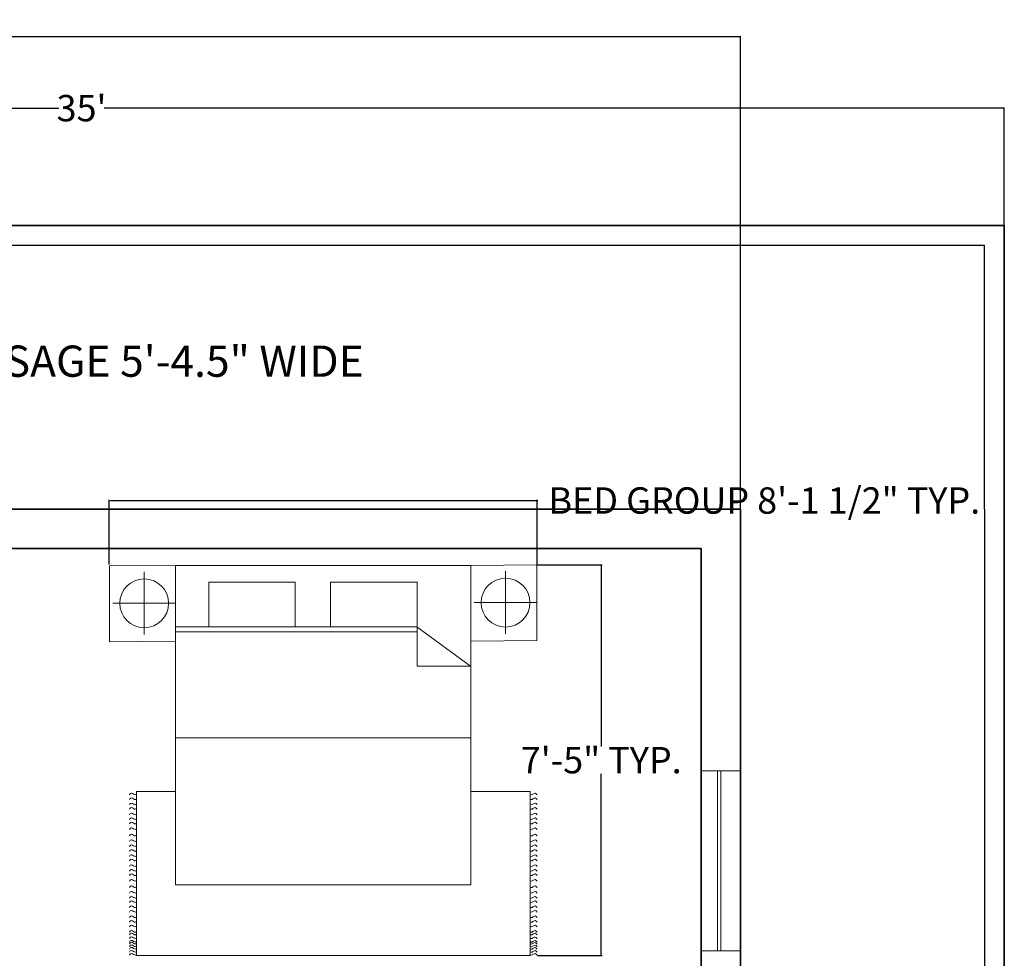
# Model space of a CAD drawing. Units: inches. Extents: x 79 to 8696167, y -3690578 to 147.
# Tile 7 of 10: x 329 to 553, y -67 to 147. Entities that reach past the tile are written whole.
import ezdxf

# ---------------------------------------------------------------- set-up
doc = ezdxf.new("R2010")
doc.units = ezdxf.units.IN
doc.header["$MEASUREMENT"] = 0
doc.layers.get('0').update_dxf_attribs({"color": 253})
for name, color, linetype, lineweight in [('A-ANNO-DIMS', 2, 'Continuous', 18), ('A-AREA-IDEN', 7, 'Continuous', 18), ('C-PROP', 7, 'Continuous', 35), ('C-SITE-WALL', 8, 'Continuous', 25), ('furniture', 30, 'Continuous', 18), ('walls', 8, 'Continuous', 35), ('windows', 171, 'Continuous', 18)]:
    doc.layers.add(name, color=color, linetype=linetype, lineweight=lineweight)
doc.styles.get("Standard").update_dxf_attribs({"font": 'arial.ttf'})
doc.dimstyles.get("Standard").update_dxf_attribs({"dimtxt": 6, "dimasz": 0.18, "dimexe": 0.18, "dimexo": 0.0625, "dimgap": 0.09, "dimtad": 0, "dimtih": 1, "dimtoh": 1, "dimzin": 0, "dimdsep": 46, "dimlunit": 3, "dimtxsty": 'Standard', "dimcen": 0.09, "dimadec": 0, "dimazin": 0, "dimtfac": 1, "dimtofl": 0, "dimtmove": 0, "dimatfit": 3, "dimfxl": 1, "dimtolj": 1, "dimtzin": 0, "dimarcsym": 0})

# ---------------------------------------------------------------- blocks, each defined once
blk = doc.blocks.new('CARPET')
at = {"layer": 'furniture'}
for p, q in [((-51.53, -98.11), (-51.53, -55.12)), ((-51.53, -55.12), (-41.27, -55.12)), ((36, -55.12), (51.55, -55.12)), ((51.55, -55.12), (51.55, -98.11)), ((51.55, -98.11), (-51.53, -98.11))]:
    blk.add_line(p, q, dxfattribs=at)
for points, knots in [([(-53.37, -55.99), (-53.22, -55.8), (-52.9, -55.41), (-52.34, -55.8), (-51.89, -56.08), (-51.65, -55.91), (-51.53, -55.83)], [0, 0, 0, 0, 0.653278, 1.290138, 1.740457, 2.114451, 2.114451, 2.114451, 2.114451]), ([(53.37, -55.99), (53.22, -55.8), (52.9, -55.41), (52.34, -55.8), (51.89, -56.08), (51.65, -55.91), (51.53, -55.83)], [0, 0, 0, 0, 0.653278, 1.290138, 1.740457, 2.114451, 2.114451, 2.114451, 2.114451]), ([(-53.37, -57.26), (-53.22, -57.07), (-52.9, -56.67), (-52.34, -57.07), (-51.89, -57.35), (-51.65, -57.17), (-51.53, -57.1)], [0, 0, 0, 0, 0.653278, 1.290138, 1.740457, 2.114451, 2.114451, 2.114451, 2.114451]), ([(-53.37, -58.59), (-53.22, -58.4), (-52.9, -58.01), (-52.34, -58.4), (-51.89, -58.68), (-51.65, -58.5), (-51.53, -58.43)], [0, 0, 0, 0, 0.653278, 1.290138, 1.740457, 2.114451, 2.114451, 2.114451, 2.114451]), ([(53.37, -57.26), (53.22, -57.07), (52.9, -56.67), (52.34, -57.07), (51.89, -57.35), (51.65, -57.17), (51.53, -57.1)], [0, 0, 0, 0, 0.653278, 1.290138, 1.740457, 2.114451, 2.114451, 2.114451, 2.114451]), ([(53.37, -58.59), (53.22, -58.4), (52.9, -58.01), (52.34, -58.4), (51.89, -58.68), (51.65, -58.5), (51.53, -58.43)], [0, 0, 0, 0, 0.653278, 1.290138, 1.740457, 2.114451, 2.114451, 2.114451, 2.114451]), ([(-53.37, -59.78), (-53.22, -59.58), (-52.9, -59.19), (-52.34, -59.58), (-51.89, -59.86), (-51.65, -59.69), (-51.53, -59.61)], [0, 0, 0, 0, 0.653278, 1.290138, 1.740457, 2.114451, 2.114451, 2.114451, 2.114451]), ([(-53.37, -61.22), (-53.22, -61.02), (-52.9, -60.63), (-52.34, -61.02), (-51.89, -61.3), (-51.65, -61.13), (-51.53, -61.05)], [0, 0, 0, 0, 0.653278, 1.290138, 1.740457, 2.114451, 2.114451, 2.114451, 2.114451]), ([(53.37, -59.78), (53.22, -59.58), (52.9, -59.19), (52.34, -59.58), (51.89, -59.86), (51.65, -59.69), (51.53, -59.61)], [0, 0, 0, 0, 0.653278, 1.290138, 1.740457, 2.114451, 2.114451, 2.114451, 2.114451]), ([(53.37, -61.22), (53.22, -61.02), (52.9, -60.63), (52.34, -61.02), (51.89, -61.3), (51.65, -61.13), (51.53, -61.05)], [0, 0, 0, 0, 0.653278, 1.290138, 1.740457, 2.114451, 2.114451, 2.114451, 2.114451]), ([(-53.37, -62.44), (-53.22, -62.25), (-52.9, -61.86), (-52.34, -62.25), (-51.89, -62.53), (-51.65, -62.36), (-51.53, -62.28)], [0, 0, 0, 0, 0.653278, 1.290138, 1.740457, 2.114451, 2.114451, 2.114451, 2.114451]), ([(-53.37, -63.63), (-53.22, -63.43), (-52.9, -63.04), (-52.34, -63.43), (-51.89, -63.72), (-51.65, -63.54), (-51.53, -63.46)], [0, 0, 0, 0, 0.653278, 1.290138, 1.740457, 2.114451, 2.114451, 2.114451, 2.114451]), ([(53.37, -62.44), (53.22, -62.25), (52.9, -61.86), (52.34, -62.25), (51.89, -62.53), (51.65, -62.36), (51.53, -62.28)], [0, 0, 0, 0, 0.653278, 1.290138, 1.740457, 2.114451, 2.114451, 2.114451, 2.114451]), ([(53.37, -63.63), (53.22, -63.43), (52.9, -63.04), (52.34, -63.43), (51.89, -63.72), (51.65, -63.54), (51.53, -63.46)], [0, 0, 0, 0, 0.653278, 1.290138, 1.740457, 2.114451, 2.114451, 2.114451, 2.114451]), ([(-53.37, -65.07), (-53.22, -64.87), (-52.9, -64.48), (-52.34, -64.87), (-51.89, -65.15), (-51.65, -64.98), (-51.53, -64.9)], [0, 0, 0, 0, 0.653278, 1.290138, 1.740457, 2.114451, 2.114451, 2.114451, 2.114451]), ([(-53.37, -66.76), (-53.22, -66.56), (-52.9, -66.17), (-52.34, -66.56), (-51.89, -66.84), (-51.65, -66.67), (-51.53, -66.59)], [0, 0, 0, 0, 0.653278, 1.290138, 1.740457, 2.114451, 2.114451, 2.114451, 2.114451]), ([(53.37, -65.07), (53.22, -64.87), (52.9, -64.48), (52.34, -64.87), (51.89, -65.15), (51.65, -64.98), (51.53, -64.9)], [0, 0, 0, 0, 0.653278, 1.290138, 1.740457, 2.114451, 2.114451, 2.114451, 2.114451]), ([(53.37, -66.76), (53.22, -66.56), (52.9, -66.17), (52.34, -66.56), (51.89, -66.84), (51.65, -66.67), (51.53, -66.59)], [0, 0, 0, 0, 0.653278, 1.290138, 1.740457, 2.114451, 2.114451, 2.114451, 2.114451]), ([(-53.37, -68.2), (-53.22, -68), (-52.9, -67.61), (-52.34, -68), (-51.89, -68.28), (-51.65, -68.11), (-51.53, -68.03)], [0, 0, 0, 0, 0.653278, 1.290138, 1.740457, 2.114451, 2.114451, 2.114451, 2.114451]), ([(-53.37, -69.53), (-53.22, -69.33), (-52.9, -68.94), (-52.34, -69.33), (-51.89, -69.61), (-51.65, -69.44), (-51.53, -69.36)], [0, 0, 0, 0, 0.653278, 1.290138, 1.740457, 2.114451, 2.114451, 2.114451, 2.114451]), ([(53.37, -68.2), (53.22, -68), (52.9, -67.61), (52.34, -68), (51.89, -68.28), (51.65, -68.11), (51.53, -68.03)], [0, 0, 0, 0, 0.653278, 1.290138, 1.740457, 2.114451, 2.114451, 2.114451, 2.114451]), ([(53.37, -69.53), (53.22, -69.33), (52.9, -68.94), (52.34, -69.33), (51.89, -69.61), (51.65, -69.44), (51.53, -69.36)], [0, 0, 0, 0, 0.653278, 1.290138, 1.740457, 2.114451, 2.114451, 2.114451, 2.114451]), ([(-53.37, -70.79), (-53.22, -70.6), (-52.9, -70.21), (-52.34, -70.6), (-51.89, -70.88), (-51.65, -70.7), (-51.53, -70.63)], [0, 0, 0, 0, 0.653278, 1.290138, 1.740457, 2.114451, 2.114451, 2.114451, 2.114451]), ([(-53.37, -72.12), (-53.22, -71.93), (-52.9, -71.54), (-52.34, -71.93), (-51.89, -72.21), (-51.65, -72.04), (-51.53, -71.96)], [0, 0, 0, 0, 0.653278, 1.290138, 1.740457, 2.114451, 2.114451, 2.114451, 2.114451]), ([(53.37, -70.79), (53.22, -70.6), (52.9, -70.21), (52.34, -70.6), (51.89, -70.88), (51.65, -70.7), (51.53, -70.63)], [0, 0, 0, 0, 0.653278, 1.290138, 1.740457, 2.114451, 2.114451, 2.114451, 2.114451]), ([(53.37, -72.12), (53.22, -71.93), (52.9, -71.54), (52.34, -71.93), (51.89, -72.21), (51.65, -72.04), (51.53, -71.96)], [0, 0, 0, 0, 0.653278, 1.290138, 1.740457, 2.114451, 2.114451, 2.114451, 2.114451]), ([(-53.37, -73.31), (-53.22, -73.11), (-52.9, -72.72), (-52.34, -73.11), (-51.89, -73.4), (-51.65, -73.22), (-51.53, -73.14)], [0, 0, 0, 0, 0.653278, 1.290138, 1.740457, 2.114451, 2.114451, 2.114451, 2.114451]), ([(-53.37, -74.75), (-53.22, -74.55), (-52.9, -74.16), (-52.34, -74.55), (-51.89, -74.83), (-51.65, -74.66), (-51.53, -74.58)], [0, 0, 0, 0, 0.653278, 1.290138, 1.740457, 2.114451, 2.114451, 2.114451, 2.114451]), ([(53.37, -73.31), (53.22, -73.11), (52.9, -72.72), (52.34, -73.11), (51.89, -73.4), (51.65, -73.22), (51.53, -73.14)], [0, 0, 0, 0, 0.653278, 1.290138, 1.740457, 2.114451, 2.114451, 2.114451, 2.114451]), ([(53.37, -74.75), (53.22, -74.55), (52.9, -74.16), (52.34, -74.55), (51.89, -74.83), (51.65, -74.66), (51.53, -74.58)], [0, 0, 0, 0, 0.653278, 1.290138, 1.740457, 2.114451, 2.114451, 2.114451, 2.114451]), ([(-53.37, -75.98), (-53.22, -75.78), (-52.9, -75.39), (-52.34, -75.78), (-51.89, -76.06), (-51.65, -75.89), (-51.53, -75.81)], [0, 0, 0, 0, 0.653278, 1.290138, 1.740457, 2.114451, 2.114451, 2.114451, 2.114451]), ([(-53.37, -77.16), (-53.22, -76.96), (-52.9, -76.57), (-52.34, -76.96), (-51.89, -77.25), (-51.65, -77.07), (-51.53, -76.99)], [0, 0, 0, 0, 0.653278, 1.290138, 1.740457, 2.114451, 2.114451, 2.114451, 2.114451]), ([(53.37, -75.98), (53.22, -75.78), (52.9, -75.39), (52.34, -75.78), (51.89, -76.06), (51.65, -75.89), (51.53, -75.81)], [0, 0, 0, 0, 0.653278, 1.290138, 1.740457, 2.114451, 2.114451, 2.114451, 2.114451]), ([(53.37, -77.16), (53.22, -76.96), (52.9, -76.57), (52.34, -76.96), (51.89, -77.25), (51.65, -77.07), (51.53, -76.99)], [0, 0, 0, 0, 0.653278, 1.290138, 1.740457, 2.114451, 2.114451, 2.114451, 2.114451]), ([(-53.37, -78.6), (-53.22, -78.4), (-52.9, -78.01), (-52.34, -78.4), (-51.89, -78.68), (-51.65, -78.51), (-51.53, -78.43)], [0, 0, 0, 0, 0.653278, 1.290138, 1.740457, 2.114451, 2.114451, 2.114451, 2.114451]), ([(-53.37, -80.29), (-53.22, -80.09), (-52.9, -79.7), (-52.34, -80.09), (-51.89, -80.37), (-51.65, -80.2), (-51.53, -80.12)], [0, 0, 0, 0, 0.653278, 1.290138, 1.740457, 2.114451, 2.114451, 2.114451, 2.114451]), ([(53.37, -78.6), (53.22, -78.4), (52.9, -78.01), (52.34, -78.4), (51.89, -78.68), (51.65, -78.51), (51.53, -78.43)], [0, 0, 0, 0, 0.653278, 1.290138, 1.740457, 2.114451, 2.114451, 2.114451, 2.114451]), ([(53.37, -80.29), (53.22, -80.09), (52.9, -79.7), (52.34, -80.09), (51.89, -80.37), (51.65, -80.2), (51.53, -80.12)], [0, 0, 0, 0, 0.653278, 1.290138, 1.740457, 2.114451, 2.114451, 2.114451, 2.114451]), ([(-53.37, -81.73), (-53.22, -81.53), (-52.9, -81.14), (-52.34, -81.53), (-51.89, -81.81), (-51.65, -81.64), (-51.53, -81.56)], [0, 0, 0, 0, 0.653278, 1.290138, 1.740457, 2.114451, 2.114451, 2.114451, 2.114451]), ([(53.37, -81.73), (53.22, -81.53), (52.9, -81.14), (52.34, -81.53), (51.89, -81.81), (51.65, -81.64), (51.53, -81.56)], [0, 0, 0, 0, 0.653278, 1.290138, 1.740457, 2.114451, 2.114451, 2.114451, 2.114451]), ([(-53.37, -83.06), (-53.22, -82.86), (-52.9, -82.47), (-52.34, -82.86), (-51.89, -83.14), (-51.65, -82.97), (-51.53, -82.89)], [0, 0, 0, 0, 0.653278, 1.290138, 1.740457, 2.114451, 2.114451, 2.114451, 2.114451]), ([(-53.37, -84.18), (-53.22, -83.99), (-52.9, -83.6), (-52.34, -83.99), (-51.89, -84.27), (-51.65, -84.09), (-51.53, -84.02)], [0, 0, 0, 0, 0.653278, 1.290138, 1.740457, 2.114451, 2.114451, 2.114451, 2.114451]), ([(-53.37, -85.51), (-53.22, -85.32), (-52.9, -84.93), (-52.34, -85.32), (-51.89, -85.6), (-51.65, -85.42), (-51.53, -85.35)], [0, 0, 0, 0, 0.653278, 1.290138, 1.740457, 2.114451, 2.114451, 2.114451, 2.114451]), ([(53.37, -83.06), (53.22, -82.86), (52.9, -82.47), (52.34, -82.86), (51.89, -83.14), (51.65, -82.97), (51.53, -82.89)], [0, 0, 0, 0, 0.653278, 1.290138, 1.740457, 2.114451, 2.114451, 2.114451, 2.114451]), ([(53.37, -84.18), (53.22, -83.99), (52.9, -83.6), (52.34, -83.99), (51.89, -84.27), (51.65, -84.09), (51.53, -84.02)], [0, 0, 0, 0, 0.653278, 1.290138, 1.740457, 2.114451, 2.114451, 2.114451, 2.114451]), ([(53.37, -85.51), (53.22, -85.32), (52.9, -84.93), (52.34, -85.32), (51.89, -85.6), (51.65, -85.42), (51.53, -85.35)], [0, 0, 0, 0, 0.653278, 1.290138, 1.740457, 2.114451, 2.114451, 2.114451, 2.114451]), ([(-53.37, -86.7), (-53.22, -86.5), (-52.9, -86.11), (-52.34, -86.5), (-51.89, -86.78), (-51.65, -86.61), (-51.53, -86.53)], [0, 0, 0, 0, 0.653278, 1.290138, 1.740457, 2.114451, 2.114451, 2.114451, 2.114451]), ([(53.37, -86.7), (53.22, -86.5), (52.9, -86.11), (52.34, -86.5), (51.89, -86.78), (51.65, -86.61), (51.53, -86.53)], [0, 0, 0, 0, 0.653278, 1.290138, 1.740457, 2.114451, 2.114451, 2.114451, 2.114451]), ([(-53.37, -88.14), (-53.22, -87.94), (-52.9, -87.55), (-52.34, -87.94), (-51.89, -88.22), (-51.65, -88.05), (-51.53, -87.97)], [0, 0, 0, 0, 0.653278, 1.290138, 1.740457, 2.114451, 2.114451, 2.114451, 2.114451]), ([(-53.37, -89.36), (-53.22, -89.17), (-52.9, -88.78), (-52.34, -89.17), (-51.89, -89.45), (-51.65, -89.28), (-51.53, -89.2)], [0, 0, 0, 0, 0.653278, 1.290138, 1.740457, 2.114451, 2.114451, 2.114451, 2.114451]), ([(-53.37, -90.55), (-53.22, -90.35), (-52.9, -89.96), (-52.34, -90.35), (-51.89, -90.64), (-51.65, -90.46), (-51.53, -90.38)], [0, 0, 0, 0, 0.653278, 1.290138, 1.740457, 2.114451, 2.114451, 2.114451, 2.114451]), ([(53.37, -88.14), (53.22, -87.94), (52.9, -87.55), (52.34, -87.94), (51.89, -88.22), (51.65, -88.05), (51.53, -87.97)], [0, 0, 0, 0, 0.653278, 1.290138, 1.740457, 2.114451, 2.114451, 2.114451, 2.114451]), ([(53.37, -89.36), (53.22, -89.17), (52.9, -88.78), (52.34, -89.17), (51.89, -89.45), (51.65, -89.28), (51.53, -89.2)], [0, 0, 0, 0, 0.653278, 1.290138, 1.740457, 2.114451, 2.114451, 2.114451, 2.114451]), ([(53.37, -90.55), (53.22, -90.35), (52.9, -89.96), (52.34, -90.35), (51.9, -90.63), (51.66, -90.47), (51.55, -90.4)], [0, 0, 0, 0, 0.653278, 1.290138, 1.740457, 2.0926, 2.0926, 2.0926, 2.0926]), ([(-53.37, -91.99), (-53.22, -91.79), (-52.9, -91.4), (-52.34, -91.79), (-51.89, -92.07), (-51.65, -91.9), (-51.53, -91.82)], [0, 0, 0, 0, 0.653278, 1.290138, 1.740457, 2.114451, 2.114451, 2.114451, 2.114451]), ([(-53.37, -92.69), (-53.22, -92.48), (-52.9, -92.08), (-52.35, -92.49), (-51.89, -92.77), (-51.65, -92.6), (-51.53, -92.52)], [0, 0, 0, 0, 0.663904, 1.307406, 1.757725, 2.131719, 2.131719, 2.131719, 2.131719]), ([(53.37, -91.99), (53.22, -91.79), (52.9, -91.4), (52.34, -91.79), (51.9, -92.07), (51.66, -91.91), (51.55, -91.83)], [0, 0, 0, 0, 0.653278, 1.290138, 1.740457, 2.0926, 2.0926, 2.0926, 2.0926]), ([(53.37, -92.69), (53.22, -92.49), (52.9, -92.09), (52.34, -92.49), (51.9, -92.77), (51.66, -92.61), (51.55, -92.53)], [0, 0, 0, 0, 0.656792, 1.295826, 1.746145, 2.098292, 2.098292, 2.098292, 2.098292]), ([(-53.37, -93.61), (-53.22, -93.42), (-52.9, -93.03), (-52.34, -93.42), (-51.89, -93.7), (-51.65, -93.52), (-51.53, -93.45)], [0, 0, 0, 0, 0.653278, 1.290138, 1.740457, 2.114451, 2.114451, 2.114451, 2.114451]), ([(-53.37, -94.55), (-53.22, -94.35), (-52.9, -93.96), (-52.34, -94.35), (-51.89, -94.63), (-51.65, -94.46), (-51.53, -94.38)], [0, 0, 0, 0, 0.653278, 1.290138, 1.740457, 2.114451, 2.114451, 2.114451, 2.114451]), ([(-53.37, -95.05), (-53.22, -94.85), (-52.9, -94.46), (-52.34, -94.85), (-51.89, -95.14), (-51.65, -94.96), (-51.53, -94.88)], [0, 0, 0, 0, 0.653278, 1.290138, 1.740457, 2.114451, 2.114451, 2.114451, 2.114451]), ([(-53.37, -95.73), (-53.22, -95.54), (-52.9, -95.15), (-52.34, -95.54), (-51.89, -95.82), (-51.65, -95.65), (-51.53, -95.57)], [0, 0, 0, 0, 0.653278, 1.290138, 1.740457, 2.114451, 2.114451, 2.114451, 2.114451]), ([(53.37, -95.78), (53.22, -95.58), (52.9, -95.19), (52.34, -95.58), (51.89, -95.86), (51.65, -95.69), (51.53, -95.61)], [0, 0, 0, 0, 0.653278, 1.290138, 1.740457, 2.114451, 2.114451, 2.114451, 2.114451]), ([(53.37, -93.66), (53.22, -93.46), (52.9, -93.07), (52.34, -93.46), (51.9, -93.74), (51.66, -93.58), (51.55, -93.5)], [0, 0, 0, 0, 0.653278, 1.290138, 1.740457, 2.0926, 2.0926, 2.0926, 2.0926]), ([(53.37, -94.59), (53.22, -94.4), (52.9, -94.01), (52.34, -94.4), (51.9, -94.68), (51.66, -94.51), (51.55, -94.44)], [0, 0, 0, 0, 0.653278, 1.290138, 1.740457, 2.0926, 2.0926, 2.0926, 2.0926]), ([(53.37, -95.1), (53.22, -94.9), (52.9, -94.51), (52.34, -94.9), (51.9, -95.18), (51.66, -95.02), (51.55, -94.94)], [0, 0, 0, 0, 0.653278, 1.290138, 1.740457, 2.0926, 2.0926, 2.0926, 2.0926]), ([(-53.37, -96.38), (-53.22, -96.18), (-52.9, -95.79), (-52.34, -96.18), (-51.89, -96.47), (-51.65, -96.29), (-51.53, -96.21)], [0, 0, 0, 0, 0.653278, 1.290138, 1.740457, 2.114451, 2.114451, 2.114451, 2.114451]), ([(-53.37, -97.17), (-53.22, -96.98), (-52.9, -96.59), (-52.34, -96.98), (-51.89, -97.26), (-51.65, -97.08), (-51.53, -97.01)], [0, 0, 0, 0, 0.653278, 1.290138, 1.740457, 2.114451, 2.114451, 2.114451, 2.114451]), ([(-53.37, -97.99), (-53.22, -97.79), (-52.9, -97.4), (-52.34, -97.79), (-51.89, -98.08), (-51.65, -97.9), (-51.53, -97.82)], [0, 0, 0, 0, 0.653278, 1.290138, 1.740457, 2.114451, 2.114451, 2.114451, 2.114451]), ([(53.37, -96.43), (53.22, -96.23), (52.9, -95.84), (52.34, -96.23), (51.89, -96.51), (51.65, -96.34), (51.53, -96.26)], [0, 0, 0, 0, 0.653278, 1.290138, 1.740457, 2.114451, 2.114451, 2.114451, 2.114451]), ([(53.37, -97.22), (53.22, -97.02), (52.9, -96.63), (52.34, -97.02), (51.89, -97.3), (51.65, -97.13), (51.53, -97.05)], [0, 0, 0, 0, 0.653278, 1.290138, 1.740457, 2.114451, 2.114451, 2.114451, 2.114451]), ([(53.37, -97.99), (53.22, -97.79), (52.9, -97.4), (52.34, -97.79), (51.89, -98.08), (51.65, -97.9), (51.53, -97.82)], [0, 0, 0, 0, 0.653278, 1.290138, 1.740457, 2.114451, 2.114451, 2.114451, 2.114451])]:
    blk.add_open_spline(points, degree=3, knots=knots, dxfattribs=at)
blk = doc.blocks.new('A$C58D270C6')
at = {"layer": 'furniture'}
for p, q in [((9.09, 124.13), (9.09, 108.87)), ((1.46, 116.5), (16.73, 116.5)), ((14.97, 94.84), (24.62, 107.92)), ((24.62, 94.93), (24.62, 107.92)), ((42.08, 108), (42.08, 36)), ((14.97, 94.93), (24.62, 94.93)), ((14.97, 94.84), (14.97, 36)), ((16.22, 94.93), (16.22, 36)), ((9.25, 36), (9.25, 20.74)), ((1.62, 28.37), (16.88, 28.37))]:
    blk.add_line(p, q, dxfattribs=at)
for points in [[(18.5, 108), (18.34, 124.13), (-0.16, 124.13), (0, 108)], [(0, 108), (77.91, 108), (77.91, 36), (0, 36)], [(4.09, 94.93), (14.97, 94.93), (14.97, 73.83), (4.09, 73.83)], [(4.09, 65.23), (14.97, 65.23), (14.97, 44.13), (4.09, 44.13)], [(18.65, 19.87), (18.5, 36), (0, 36), (0.16, 19.87)]]:
    blk.add_lwpolyline(points, close=True, dxfattribs=at)
for centre in [(9.09, 116.5), (9.25, 28.37)]:
    blk.add_circle(centre, 5.95, dxfattribs=at)
at = {"layer": 'furniture', "xscale": 0.9312884925094044, "yscale": 0.9312884925094044, "zscale": 0.9312884925094044, "rotation": 90}
blk.add_blockref('CARPET', (3.79, 74.47), dxfattribs=at)
blk = doc.blocks.new('*D22')
at = {"layer": 'A-ANNO-DIMS', "color": 0, "lineweight": -2, "transparency": 16777216}
for p, q in [((133.44, 99.94), (133.44, 126.77)), ((133.62, 126.59), (338.26, 126.59)), ((553.26, 126.59), (348.62, 126.59)), ((553.44, 99.94), (553.44, 126.77))]:
    blk.add_line(p, q, dxfattribs=at)
at = {"layer": 'A-ANNO-DIMS', "color": 0, "lineweight": 100, "transparency": 16777216}
for points in [[(133.62, 126.62), (133.62, 126.56), (133.44, 126.59)], [(553.26, 126.62), (553.26, 126.56), (553.44, 126.59)]]:
    blk.add_solid(points, dxfattribs=at)
at = {"layer": 'Defpoints', "color": 0, "lineweight": 100, "transparency": 16777216}
for p in [(553.44, 126.59), (133.44, 99.88), (553.44, 99.88)]:
    blk.add_point(p, dxfattribs=at)
at = {"layer": 'A-ANNO-DIMS', "color": 0, "transparency": 16777216, "insert": (343.44, 126.59), "char_height": 6, "attachment_point": 5}
blk.add_mtext("\\A1;35'", dxfattribs=at)
blk = doc.blocks.new('WIN-SIDE-41IN')
for p, q in [((0, 40.98), (9, 40.98)), ((0, 40.98), (0, 0)), ((3.73, 40.98), (3.73, 0)), ((4.5, 0), (4.5, 40.98)), ((9, 40.98), (9, 0)), ((9, 0), (0, 0))]:
    blk.add_line(p, q)
blk = doc.blocks.new('*D41')
at = {"layer": 'A-ANNO-DIMS', "color": 0, "lineweight": -2, "transparency": 16777216}
for p, q in [((349.76, 22.77), (349.76, 37.49)), ((349.94, 37.31), (446.92, 37.31)), ((447.1, 22.77), (447.1, 37.49)), ((447.1, 37.31), (447.28, 37.31))]:
    blk.add_line(p, q, dxfattribs=at)
at = {"layer": 'A-ANNO-DIMS', "color": 0, "lineweight": 100, "transparency": 16777216}
for points in [[(349.94, 37.34), (349.94, 37.28), (349.76, 37.31)], [(446.92, 37.34), (446.92, 37.28), (447.1, 37.31)]]:
    blk.add_solid(points, dxfattribs=at)
at = {"layer": 'Defpoints', "color": 0, "lineweight": 100, "transparency": 16777216}
for p in [(447.1, 37.31), (349.76, 22.71), (447.1, 22.71)]:
    blk.add_point(p, dxfattribs=at)
at = {"layer": 'A-ANNO-DIMS', "color": 0, "transparency": 16777216, "insert": (498.83, 37.31), "char_height": 6, "attachment_point": 5}
blk.add_mtext('\\A1;BED GROUP 8\'-1 1/2" TYP.', dxfattribs=at)
blk = doc.blocks.new('*D42')
at = {"layer": 'A-ANNO-DIMS', "color": 0, "lineweight": -2, "transparency": 16777216}
for p, q in [((447.17, 22.71), (461.89, 22.71)), ((461.71, 22.53), (461.71, -18.63)), ((461.71, -66.06), (461.71, -24.91)), ((447.17, -66.24), (461.89, -66.24))]:
    blk.add_line(p, q, dxfattribs=at)
at = {"layer": 'A-ANNO-DIMS', "color": 0, "lineweight": 100, "transparency": 16777216}
for points in [[(461.68, 22.53), (461.74, 22.53), (461.71, 22.71)], [(461.68, -66.06), (461.74, -66.06), (461.71, -66.24)]]:
    blk.add_solid(points, dxfattribs=at)
at = {"layer": 'Defpoints', "color": 0, "lineweight": 100, "transparency": 16777216}
for p in [(447.1, 22.71), (447.1, -66.24), (461.71, -66.24)]:
    blk.add_point(p, dxfattribs=at)
at = {"layer": 'A-ANNO-DIMS', "color": 0, "transparency": 16777216, "insert": (461.71, -21.77), "char_height": 6, "attachment_point": 5}
blk.add_mtext('\\A1;7\'-5" TYP.', dxfattribs=at)
blk = doc.blocks.new('*D55')
at = {"layer": 'A-ANNO-DIMS', "color": 0, "lineweight": -2, "transparency": 16777216}
for p, q in [((133.44, 35.44), (133.44, 142.96)), ((133.62, 142.78), (303.05, 142.78)), ((493.26, 142.78), (323.83, 142.78)), ((493.44, 35.44), (493.44, 142.96))]:
    blk.add_line(p, q, dxfattribs=at)
at = {"layer": 'A-ANNO-DIMS', "color": 0, "lineweight": 100, "transparency": 16777216}
for points in [[(133.62, 142.81), (133.62, 142.75), (133.44, 142.78)], [(493.26, 142.81), (493.26, 142.75), (493.44, 142.78)]]:
    blk.add_solid(points, dxfattribs=at)
at = {"layer": 'Defpoints', "color": 0, "lineweight": 100, "transparency": 16777216}
for p in [(493.44, 142.78), (133.44, 35.38), (493.44, 35.38)]:
    blk.add_point(p, dxfattribs=at)
at = {"layer": 'A-ANNO-DIMS', "color": 0, "transparency": 16777216, "insert": (313.44, 142.78), "char_height": 6, "attachment_point": 5}
blk.add_mtext('\\A1;30\'-0"', dxfattribs=at)

msp = doc.modelspace()

# ---------------------------------------------------------------- linework, layer by layer
at = {"layer": 'C-PROP'}
for p, q in [((133.441, 99.875), (553.441, 99.875)), ((553.441, 99.875), (553.441, -680.125))]:
    msp.add_line(p, q, dxfattribs=at)
at = {"layer": 'C-SITE-WALL'}
for p, q in [((137.941, 95.375), (548.941, 95.375)), ((548.941, 35.375), (548.941, 95.375)), ((548.941, 35.375), (548.941, -455.125))]:
    msp.add_line(p, q, dxfattribs=at)
at = {"layer": 'walls'}
for p, q in [((133.441, 35.375), (493.441, 35.375)), ((493.441, 35.375), (493.441, -455.125)), ((290.941, 26.375), (484.441, 26.375)), ((484.441, 26.375), (484.441, -107.125))]:
    msp.add_line(p, q, dxfattribs=at)

# ---------------------------------------------------------------- block references
at = {"layer": 'furniture', "xscale": 0.9331788672991836, "yscale": 0.9331788672991836, "zscale": 0.9331788672991836, "rotation": 269.9999999999999}
msp.add_blockref('A$C58D270C6', (331.222, 22.56), dxfattribs=at)
at = {"layer": 'windows'}
msp.add_blockref('WIN-SIDE-41IN', (484.441, -65.152), dxfattribs=at)

# ---------------------------------------------------------------- texts
at = {"layer": 'A-AREA-IDEN'}
msp.add_text('PASSAGE 5\'-4.5" WIDE', height=7.11297, dxfattribs=at).set_placement((308.132, 65.462))

# ---------------------------------------------------------------- dimensions: what is measured, and where the dimension line sits
at = {"layer": 'A-ANNO-DIMS'}
for base, p1, p2, override, picture, middle in [((493.441, 142.775), (133.441, 35.375), (493.441, 35.375), {"dimdec": 1, "dimlfac": 1, "dimrnd": 0, "dimzin": 1, "dimdsep": 46, "dimlunit": 4, "dimfrac": 2}, '*D55', (313.441, 142.775)), ((553.441, 126.587), (133.441, 99.875), (553.441, 99.875), {"dimclrd": 0, "dimclre": 0, "dimclrt": 0}, '*D22', (343.441, 126.587))]:
    dim = msp.add_linear_dim(base=base, p1=p1, p2=p2, dimstyle='Standard', override=override, dxfattribs=at)
    dim.commit()
    dim.dimension.update_dxf_attribs({"geometry": picture, "text_midpoint": middle})
dim = msp.add_linear_dim(base=(447.104, 37.307), p1=(349.763, 22.706), p2=(447.104, 22.706), text='BED GROUP <> TYP.', dimstyle='Standard', override={"dimdec": 1, "dimlfac": 1, "dimrnd": 0, "dimzin": 1, "dimdsep": 46, "dimlunit": 4, "dimfrac": 2}, dxfattribs=at)
dim.commit()
dim.dimension.update_dxf_attribs({"geometry": '*D41', "text_midpoint": (498.833, 37.307)})
dim = msp.add_linear_dim(base=(461.706, -66.24), p1=(447.104, 22.706), p2=(447.104, -66.24), angle=270, text='<> TYP.', dimstyle='Standard', override={"dimdec": 1, "dimlfac": 1, "dimrnd": 0, "dimzin": 1, "dimdsep": 46, "dimlunit": 4, "dimfrac": 2}, dxfattribs=at)
dim.commit()
dim.dimension.update_dxf_attribs({"geometry": '*D42', "text_midpoint": (461.706, -21.767)})

doc.saveas('drawing.dxf')
